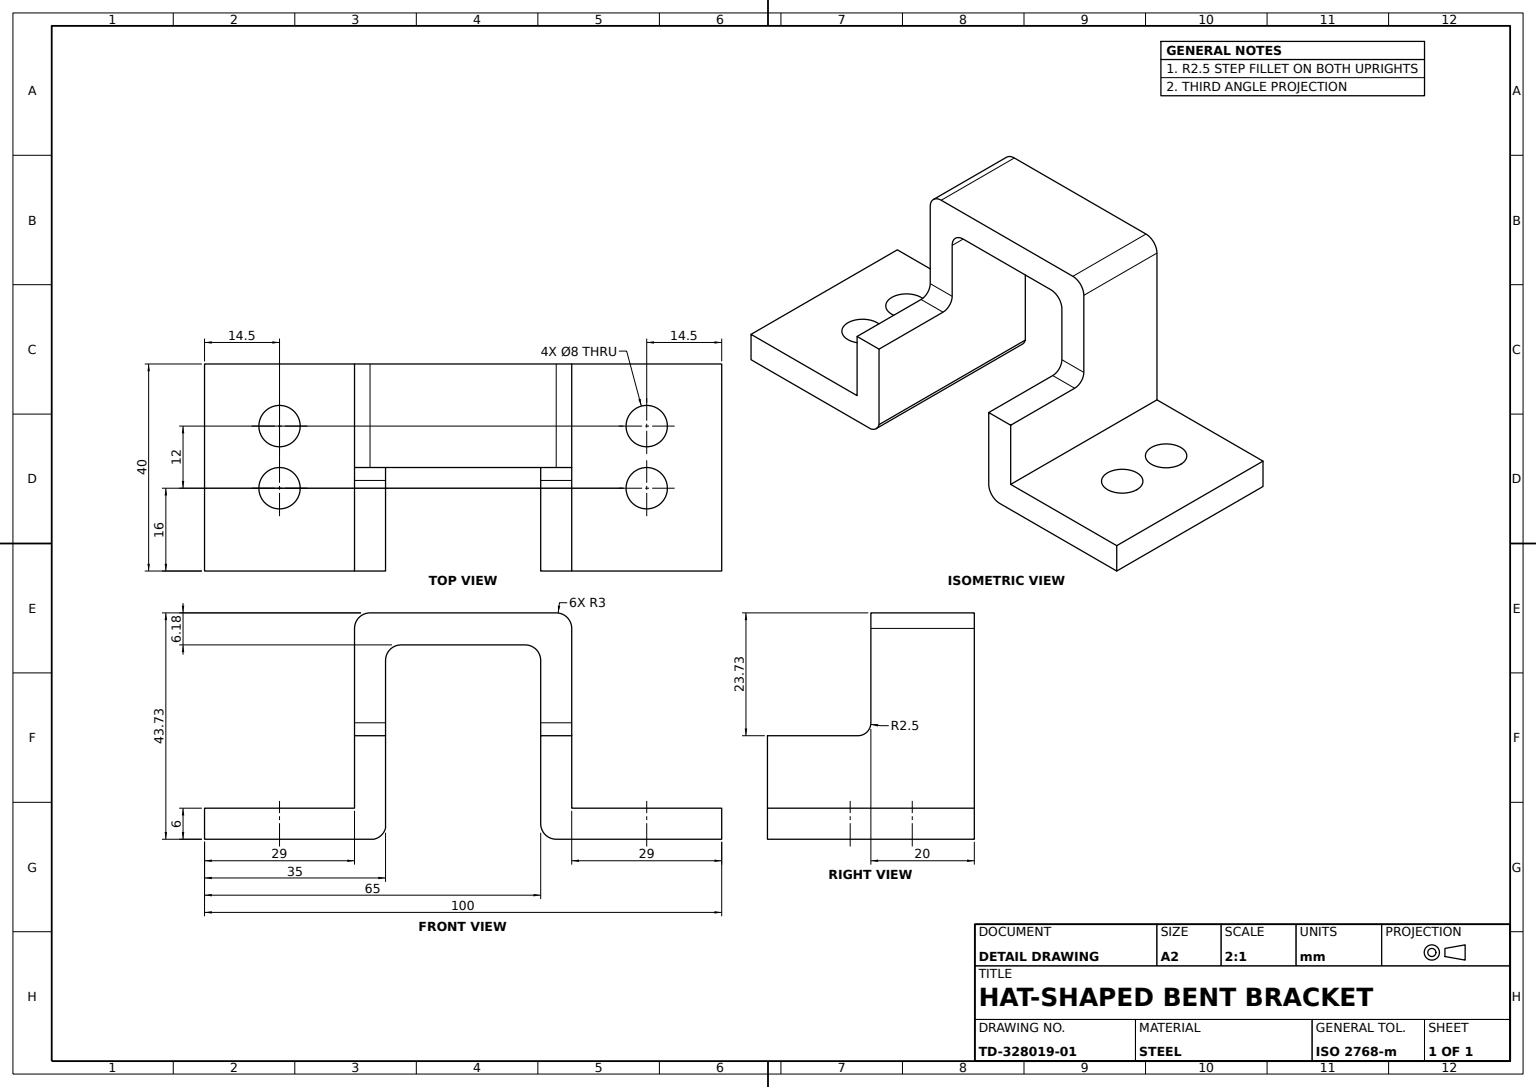
from build123d import *

# Parameters (mm, degrees)
BRACKET_BODY_40MM_DEPTH          = 20
STEPPED_START                    = 28
STEPPED_RELIEF_CUT_28MM_DEPTH    = 28
CORNER_ROUND_CUT_A_R3_DEPTH      = 88.96284726
CORNER_ROUND_CUT_B_R3_DEPTH      = 81.854576235
CORNER_ROUND_CUT_B_R3_DEPTH_BACK = 81.854576235
CORNER_FILL_BOSS_A_6MM_DEPTH     = 6
CORNER_START                     = -6
CORNER_FILL_BOSS_B_6MM_DEPTH     = 6
MOUNTING_HOLES_SKETCH_R          = 4
FLANGE_MOUNTING_HOLES_DEPTH      = 78.77327287


with BuildPart() as part:
    # Bracket Profile Sketch → Bracket Body 40mm (new, symmetric)
    with BuildSketch(Plane.XY):
        with BuildLine():
            Line((30, 0), (65, 0))
            Line((65, 0), (65, 6))
            Line((65, 6), (36, 6))
            Line((36, 6), (36, 40.731710442))
            ThreePointArc((36, 40.731710442), (35.121320344, 42.853030785), (33, 43.731710442))
            Line((33, 43.731710442), (-3, 43.731710442))
            ThreePointArc((-3, 43.731710442), (-5.121320344, 42.853030785), (-6, 40.731710442))
            Line((-6, 40.731710442), (-6, 6))
            Line((-6, 6), (-35, 6))
            Line((-35, 6), (-35, 0))
            Line((-35, 0), (0, 0))
            Line((0, 0), (0, 34.547795072))
            ThreePointArc((0, 34.547795072), (0.878679656, 36.669115416), (3, 37.547795072))
            Line((3, 37.547795072), (27, 37.547795072))
            ThreePointArc((27, 37.547795072), (29.121320344, 36.669115416), (30, 34.547795072))
            Line((30, 34.547795072), (30, 0))
        make_face()
    extrude(amount=BRACKET_BODY_40MM_DEPTH, both=True)

    # Relief Cut Sketch → Stepped Relief Cut 28mm (cut)
    with BuildSketch(Plane.XY.offset(STEPPED_START)):
        with BuildLine():
            Line((33, 43.731710442), (-3, 43.731710442))
            ThreePointArc((-3, 43.731710442), (-5.121320344, 42.853030785), (-6, 40.731710442))
            Line((-6, 40.731710442), (-6, 20))
            Line((-6, 20), (0, 20))
            Line((0, 20), (0, 34.547795072))
            ThreePointArc((0, 34.547795072), (0.878679656, 36.669115416), (3, 37.547795072))
            Line((3, 37.547795072), (27, 37.547795072))
            ThreePointArc((27, 37.547795072), (29.121320344, 36.669115416), (30, 34.547795072))
            Line((30, 34.547795072), (30, 20))
            Line((30, 20), (36, 20))
            Line((36, 20), (36, 40.731710442))
            ThreePointArc((36, 40.731710442), (35.121320344, 42.853030785), (33, 43.731710442))
        make_face()
    extrude(amount=-STEPPED_RELIEF_CUT_28MM_DEPTH, mode=Mode.SUBTRACT)

    # Corner Round Cut A Sketch → Corner Round Cut A R3 (cut, through all)
    with BuildSketch(Plane.XY.offset(20)):
        with BuildLine():
            Line((0, 2.140440117), (0, 0))
            Line((0, 0), (-2.252870035, 0))
            ThreePointArc((-2.252870035, 0), (-0.827692267, 0.755785384), (0, 2.140440117))
        make_face()
    extrude(amount=-CORNER_ROUND_CUT_A_R3_DEPTH, mode=Mode.SUBTRACT)

    # Corner Round Cut B Sketch → Corner Round Cut B R3 (cut, two sides: drawn at the far end of the back side and taken through both)
    with BuildSketch(Plane.XY.offset(-CORNER_ROUND_CUT_B_R3_DEPTH_BACK)):
        with BuildLine():
            Line((30, 0), (30, 3))
            ThreePointArc((30, 3), (30.878679656, 0.878679656), (33, 0))
            Line((33, 0), (30, 0))
        make_face()
    extrude(amount=CORNER_ROUND_CUT_B_R3_DEPTH + CORNER_ROUND_CUT_B_R3_DEPTH_BACK, mode=Mode.SUBTRACT)

    # Corner Fill Boss A Sketch → Corner Fill Boss A 6mm (add)
    with BuildSketch(Plane.ZY.offset(6)):
        with BuildLine():
            Line((0, 20), (0, 22.5))
            ThreePointArc((0, 22.5), (0.732233047, 20.732233047), (2.5, 20))
            Line((2.5, 20), (0, 20))
        make_face()
    extrude(amount=-CORNER_FILL_BOSS_A_6MM_DEPTH)

    # Corner Fill Boss B Sketch → Corner Fill Boss B 6mm (add)
    with BuildSketch(Plane(origin=(36, 0, 0), x_dir=(0, 0, -1), z_dir=(1, 0, 0)).offset(CORNER_START)):
        with BuildLine():
            Line((0, 22.5), (0, 20))
            Line((0, 20), (-2.5, 20))
            ThreePointArc((-2.5, 20), (-0.732233047, 20.732233047), (0, 22.5))
        make_face()
    extrude(amount=CORNER_FILL_BOSS_B_6MM_DEPTH)

    # Mounting Holes Sketch → Flange Mounting Holes (cut, through all)
    with BuildSketch(Plane(origin=(0, 6, 0), x_dir=(1, 0, 0), z_dir=(0, 1, 0))):
        with Locations(Location((50.5, -4, 0), (0, 0, 180))):
            Circle(MOUNTING_HOLES_SKETCH_R)
        with Locations(Location((50.5, 8, 0), (0, 0, 180))):
            Circle(MOUNTING_HOLES_SKETCH_R)
        with Locations((-20.5, -4)):
            Circle(MOUNTING_HOLES_SKETCH_R)
        with Locations((-20.5, 8)):
            Circle(MOUNTING_HOLES_SKETCH_R)
    extrude(amount=-FLANGE_MOUNTING_HOLES_DEPTH, mode=Mode.SUBTRACT)


solid = part.part
